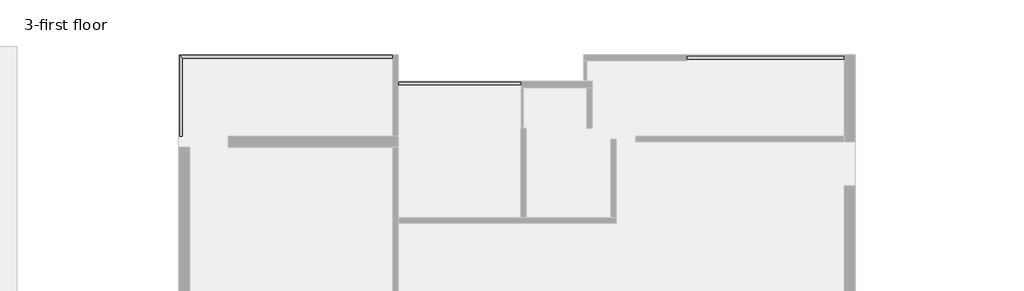
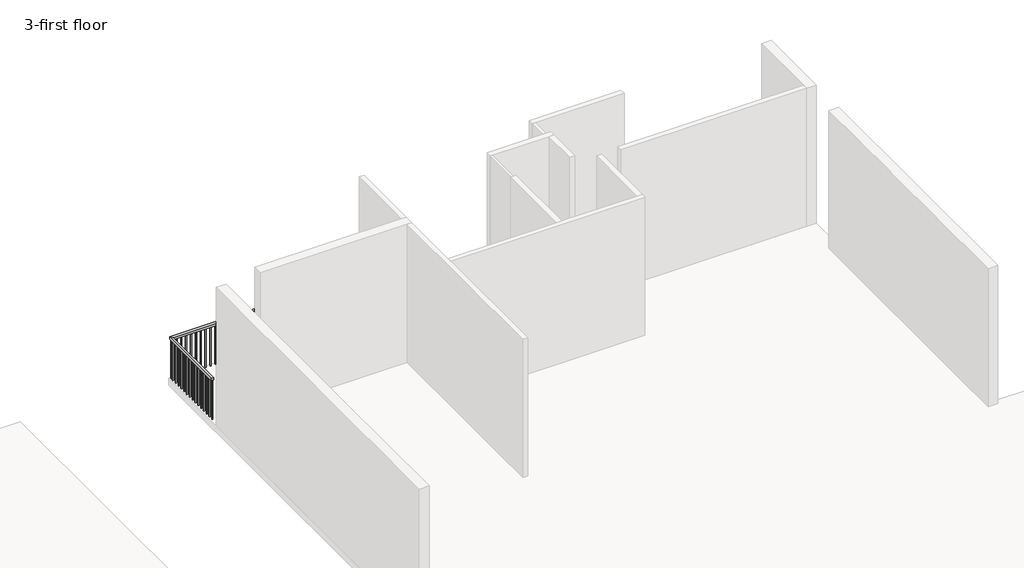
# One storey, part 2 of 2: 3 railings.
"""IFC4 building model written with IfcOpenShell, lengths in millimetres."""

from ifc_helpers import new_model, si_unit, frame, origin, place, context, project, spatial, polyline, outline, extrude, faceted_brep, element, save

model = new_model("IFC4")

# Units and contexts
model_context = context("Model", 3, world=origin())
ifc_project = project(units=[si_unit("LENGTHUNIT", "METRE", prefix="MILLI")], contexts=[model_context])

# Site, building, storey
site = spatial("IfcSite", under=ifc_project)
building = spatial("IfcBuilding", under=site)
storey = spatial("IfcBuildingStorey", under=building, Name="3-first floor", Elevation=3505.2)

# Railings
placement = place(None, origin())
element("IfcRailing", 1, ObjectType="Handrail - Rectangular", at=placement, inside=storey, context=model_context, shape_type="SolidModel", body=[
    faceted_brep([(-27068.2159189, 48850.883515, 4419.6), (-27068.2159189, 48850.883515, 4368.8), (-27017.4159189, 48850.883515, 4368.8), (-27017.4159189, 48850.883515, 4419.6), (-27017.4159189, 50306.2625405, 4368.8), (-27017.4159189, 50306.2625405, 4419.6), (-27068.2159189, 50357.0625405, 4419.6), (-23067.7159175, 50357.0625405, 4419.6), (-23067.7159175, 50306.2625405, 4419.6), (-23067.7159175, 50306.2625405, 4368.8), (-23067.7159175, 50357.0625405, 4368.8), (-27068.2159189, 50357.0625405, 4368.8)], [[[0, 1, 2, 3]], [[3, 2, 4, 5]], [[0, 3, 5, 6]], [[7, 8, 9, 10]], [[5, 4, 9, 8]], [[6, 5, 8, 7]], [[1, 0, 6, 11]], [[2, 1, 11, 4]], [[11, 6, 7, 10]], [[4, 11, 10, 9]]]),
    extrude(outline(polyline([(-23089.9409189, 50322.1375405), (-23089.9409189, 50341.1875405), (-23070.8909189, 50341.1875405), (-23070.8909189, 50322.1375405), (-23089.9409189, 50322.1375405)])), frame((0.0, 0.0, 3505.2), z_axis=(0.0, 0.0, 1.0), x_axis=(1.0, 0.0, 0.0)), (0.0, 0.0, 1.0), 863.6),
    extrude(outline(polyline([(-23191.5409189, 50322.1375405), (-23191.5409189, 50341.1875405), (-23172.4909189, 50341.1875405), (-23172.4909189, 50322.1375405), (-23191.5409189, 50322.1375405)])), frame((0.0, 0.0, 3505.2), z_axis=(0.0, 0.0, 1.0), x_axis=(1.0, 0.0, 0.0)), (0.0, 0.0, 1.0), 863.6),
    extrude(outline(polyline([(-23293.1409189, 50322.1375405), (-23293.1409189, 50341.1875405), (-23274.0909189, 50341.1875405), (-23274.0909189, 50322.1375405), (-23293.1409189, 50322.1375405)])), frame((0.0, 0.0, 3505.2), z_axis=(0.0, 0.0, 1.0), x_axis=(1.0, 0.0, 0.0)), (0.0, 0.0, 1.0), 863.6),
    extrude(outline(polyline([(-23394.7409189, 50322.1375405), (-23394.7409189, 50341.1875405), (-23375.6909189, 50341.1875405), (-23375.6909189, 50322.1375405), (-23394.7409189, 50322.1375405)])), frame((0.0, 0.0, 3505.2), z_axis=(0.0, 0.0, 1.0), x_axis=(1.0, 0.0, 0.0)), (0.0, 0.0, 1.0), 863.6),
    extrude(outline(polyline([(-23496.3409189, 50322.1375405), (-23496.3409189, 50341.1875405), (-23477.2909189, 50341.1875405), (-23477.2909189, 50322.1375405), (-23496.3409189, 50322.1375405)])), frame((0.0, 0.0, 3505.2), z_axis=(0.0, 0.0, 1.0), x_axis=(1.0, 0.0, 0.0)), (0.0, 0.0, 1.0), 863.6),
    extrude(outline(polyline([(-23597.9409189, 50322.1375405), (-23597.9409189, 50341.1875405), (-23578.8909189, 50341.1875405), (-23578.8909189, 50322.1375405), (-23597.9409189, 50322.1375405)])), frame((0.0, 0.0, 3505.2), z_axis=(0.0, 0.0, 1.0), x_axis=(1.0, 0.0, 0.0)), (0.0, 0.0, 1.0), 863.6),
    extrude(outline(polyline([(-23699.5409189, 50322.1375405), (-23699.5409189, 50341.1875405), (-23680.4909189, 50341.1875405), (-23680.4909189, 50322.1375405), (-23699.5409189, 50322.1375405)])), frame((0.0, 0.0, 3505.2), z_axis=(0.0, 0.0, 1.0), x_axis=(1.0, 0.0, 0.0)), (0.0, 0.0, 1.0), 863.6),
    extrude(outline(polyline([(-23801.1409189, 50322.1375405), (-23801.1409189, 50341.1875405), (-23782.0909189, 50341.1875405), (-23782.0909189, 50322.1375405), (-23801.1409189, 50322.1375405)])), frame((0.0, 0.0, 3505.2), z_axis=(0.0, 0.0, 1.0), x_axis=(1.0, 0.0, 0.0)), (0.0, 0.0, 1.0), 863.6),
    extrude(outline(polyline([(-23902.7409189, 50322.1375405), (-23902.7409189, 50341.1875405), (-23883.6909189, 50341.1875405), (-23883.6909189, 50322.1375405), (-23902.7409189, 50322.1375405)])), frame((0.0, 0.0, 3505.2), z_axis=(0.0, 0.0, 1.0), x_axis=(1.0, 0.0, 0.0)), (0.0, 0.0, 1.0), 863.6),
    extrude(outline(polyline([(-24004.3409189, 50322.1375405), (-24004.3409189, 50341.1875405), (-23985.2909189, 50341.1875405), (-23985.2909189, 50322.1375405), (-24004.3409189, 50322.1375405)])), frame((0.0, 0.0, 3505.2), z_axis=(0.0, 0.0, 1.0), x_axis=(1.0, 0.0, 0.0)), (0.0, 0.0, 1.0), 863.6),
    extrude(outline(polyline([(-24105.9409189, 50322.1375405), (-24105.9409189, 50341.1875405), (-24086.8909189, 50341.1875405), (-24086.8909189, 50322.1375405), (-24105.9409189, 50322.1375405)])), frame((0.0, 0.0, 3505.2), z_axis=(0.0, 0.0, 1.0), x_axis=(1.0, 0.0, 0.0)), (0.0, 0.0, 1.0), 863.6),
    extrude(outline(polyline([(-24207.5409189, 50322.1375405), (-24207.5409189, 50341.1875405), (-24188.4909189, 50341.1875405), (-24188.4909189, 50322.1375405), (-24207.5409189, 50322.1375405)])), frame((0.0, 0.0, 3505.2), z_axis=(0.0, 0.0, 1.0), x_axis=(1.0, 0.0, 0.0)), (0.0, 0.0, 1.0), 863.6),
    extrude(outline(polyline([(-24309.1409189, 50322.1375405), (-24309.1409189, 50341.1875405), (-24290.0909189, 50341.1875405), (-24290.0909189, 50322.1375405), (-24309.1409189, 50322.1375405)])), frame((0.0, 0.0, 3505.2), z_axis=(0.0, 0.0, 1.0), x_axis=(1.0, 0.0, 0.0)), (0.0, 0.0, 1.0), 863.6),
    extrude(outline(polyline([(-24410.7409189, 50322.1375405), (-24410.7409189, 50341.1875405), (-24391.6909189, 50341.1875405), (-24391.6909189, 50322.1375405), (-24410.7409189, 50322.1375405)])), frame((0.0, 0.0, 3505.2), z_axis=(0.0, 0.0, 1.0), x_axis=(1.0, 0.0, 0.0)), (0.0, 0.0, 1.0), 863.6),
    extrude(outline(polyline([(-24512.3409189, 50322.1375405), (-24512.3409189, 50341.1875405), (-24493.2909189, 50341.1875405), (-24493.2909189, 50322.1375405), (-24512.3409189, 50322.1375405)])), frame((0.0, 0.0, 3505.2), z_axis=(0.0, 0.0, 1.0), x_axis=(1.0, 0.0, 0.0)), (0.0, 0.0, 1.0), 863.6),
    extrude(outline(polyline([(-24613.9409189, 50322.1375405), (-24613.9409189, 50341.1875405), (-24594.8909189, 50341.1875405), (-24594.8909189, 50322.1375405), (-24613.9409189, 50322.1375405)])), frame((0.0, 0.0, 3505.2), z_axis=(0.0, 0.0, 1.0), x_axis=(1.0, 0.0, 0.0)), (0.0, 0.0, 1.0), 863.6),
    extrude(outline(polyline([(-24715.5409189, 50322.1375405), (-24715.5409189, 50341.1875405), (-24696.4909189, 50341.1875405), (-24696.4909189, 50322.1375405), (-24715.5409189, 50322.1375405)])), frame((0.0, 0.0, 3505.2), z_axis=(0.0, 0.0, 1.0), x_axis=(1.0, 0.0, 0.0)), (0.0, 0.0, 1.0), 863.6),
    extrude(outline(polyline([(-24817.1409189, 50322.1375405), (-24817.1409189, 50341.1875405), (-24798.0909189, 50341.1875405), (-24798.0909189, 50322.1375405), (-24817.1409189, 50322.1375405)])), frame((0.0, 0.0, 3505.2), z_axis=(0.0, 0.0, 1.0), x_axis=(1.0, 0.0, 0.0)), (0.0, 0.0, 1.0), 863.6),
    extrude(outline(polyline([(-24918.7409189, 50322.1375405), (-24918.7409189, 50341.1875405), (-24899.6909189, 50341.1875405), (-24899.6909189, 50322.1375405), (-24918.7409189, 50322.1375405)])), frame((0.0, 0.0, 3505.2), z_axis=(0.0, 0.0, 1.0), x_axis=(1.0, 0.0, 0.0)), (0.0, 0.0, 1.0), 863.6),
    extrude(outline(polyline([(-25020.3409189, 50322.1375405), (-25020.3409189, 50341.1875405), (-25001.2909189, 50341.1875405), (-25001.2909189, 50322.1375405), (-25020.3409189, 50322.1375405)])), frame((0.0, 0.0, 3505.2), z_axis=(0.0, 0.0, 1.0), x_axis=(1.0, 0.0, 0.0)), (0.0, 0.0, 1.0), 863.6),
    extrude(outline(polyline([(-25121.9409189, 50322.1375405), (-25121.9409189, 50341.1875405), (-25102.8909189, 50341.1875405), (-25102.8909189, 50322.1375405), (-25121.9409189, 50322.1375405)])), frame((0.0, 0.0, 3505.2), z_axis=(0.0, 0.0, 1.0), x_axis=(1.0, 0.0, 0.0)), (0.0, 0.0, 1.0), 863.6),
    extrude(outline(polyline([(-25223.5409189, 50322.1375405), (-25223.5409189, 50341.1875405), (-25204.4909189, 50341.1875405), (-25204.4909189, 50322.1375405), (-25223.5409189, 50322.1375405)])), frame((0.0, 0.0, 3505.2), z_axis=(0.0, 0.0, 1.0), x_axis=(1.0, 0.0, 0.0)), (0.0, 0.0, 1.0), 863.6),
    extrude(outline(polyline([(-25325.1409189, 50322.1375405), (-25325.1409189, 50341.1875405), (-25306.0909189, 50341.1875405), (-25306.0909189, 50322.1375405), (-25325.1409189, 50322.1375405)])), frame((0.0, 0.0, 3505.2), z_axis=(0.0, 0.0, 1.0), x_axis=(1.0, 0.0, 0.0)), (0.0, 0.0, 1.0), 863.6),
    extrude(outline(polyline([(-25426.7409189, 50322.1375405), (-25426.7409189, 50341.1875405), (-25407.6909189, 50341.1875405), (-25407.6909189, 50322.1375405), (-25426.7409189, 50322.1375405)])), frame((0.0, 0.0, 3505.2), z_axis=(0.0, 0.0, 1.0), x_axis=(1.0, 0.0, 0.0)), (0.0, 0.0, 1.0), 863.6),
    extrude(outline(polyline([(-25528.3409189, 50322.1375405), (-25528.3409189, 50341.1875405), (-25509.2909189, 50341.1875405), (-25509.2909189, 50322.1375405), (-25528.3409189, 50322.1375405)])), frame((0.0, 0.0, 3505.2), z_axis=(0.0, 0.0, 1.0), x_axis=(1.0, 0.0, 0.0)), (0.0, 0.0, 1.0), 863.6),
    extrude(outline(polyline([(-25629.9409189, 50322.1375405), (-25629.9409189, 50341.1875405), (-25610.8909189, 50341.1875405), (-25610.8909189, 50322.1375405), (-25629.9409189, 50322.1375405)])), frame((0.0, 0.0, 3505.2), z_axis=(0.0, 0.0, 1.0), x_axis=(1.0, 0.0, 0.0)), (0.0, 0.0, 1.0), 863.6),
    extrude(outline(polyline([(-25731.5409189, 50322.1375405), (-25731.5409189, 50341.1875405), (-25712.4909189, 50341.1875405), (-25712.4909189, 50322.1375405), (-25731.5409189, 50322.1375405)])), frame((0.0, 0.0, 3505.2), z_axis=(0.0, 0.0, 1.0), x_axis=(1.0, 0.0, 0.0)), (0.0, 0.0, 1.0), 863.6),
    extrude(outline(polyline([(-25833.1409189, 50322.1375405), (-25833.1409189, 50341.1875405), (-25814.0909189, 50341.1875405), (-25814.0909189, 50322.1375405), (-25833.1409189, 50322.1375405)])), frame((0.0, 0.0, 3505.2), z_axis=(0.0, 0.0, 1.0), x_axis=(1.0, 0.0, 0.0)), (0.0, 0.0, 1.0), 863.6),
    extrude(outline(polyline([(-25934.7409189, 50322.1375405), (-25934.7409189, 50341.1875405), (-25915.6909189, 50341.1875405), (-25915.6909189, 50322.1375405), (-25934.7409189, 50322.1375405)])), frame((0.0, 0.0, 3505.2), z_axis=(0.0, 0.0, 1.0), x_axis=(1.0, 0.0, 0.0)), (0.0, 0.0, 1.0), 863.6),
    extrude(outline(polyline([(-26036.3409189, 50322.1375405), (-26036.3409189, 50341.1875405), (-26017.2909189, 50341.1875405), (-26017.2909189, 50322.1375405), (-26036.3409189, 50322.1375405)])), frame((0.0, 0.0, 3505.2), z_axis=(0.0, 0.0, 1.0), x_axis=(1.0, 0.0, 0.0)), (0.0, 0.0, 1.0), 863.6),
    extrude(outline(polyline([(-26137.9409189, 50322.1375405), (-26137.9409189, 50341.1875405), (-26118.8909189, 50341.1875405), (-26118.8909189, 50322.1375405), (-26137.9409189, 50322.1375405)])), frame((0.0, 0.0, 3505.2), z_axis=(0.0, 0.0, 1.0), x_axis=(1.0, 0.0, 0.0)), (0.0, 0.0, 1.0), 863.6),
    extrude(outline(polyline([(-26239.5409189, 50322.1375405), (-26239.5409189, 50341.1875405), (-26220.4909189, 50341.1875405), (-26220.4909189, 50322.1375405), (-26239.5409189, 50322.1375405)])), frame((0.0, 0.0, 3505.2), z_axis=(0.0, 0.0, 1.0), x_axis=(1.0, 0.0, 0.0)), (0.0, 0.0, 1.0), 863.6),
    extrude(outline(polyline([(-26341.1409189, 50322.1375405), (-26341.1409189, 50341.1875405), (-26322.0909189, 50341.1875405), (-26322.0909189, 50322.1375405), (-26341.1409189, 50322.1375405)])), frame((0.0, 0.0, 3505.2), z_axis=(0.0, 0.0, 1.0), x_axis=(1.0, 0.0, 0.0)), (0.0, 0.0, 1.0), 863.6),
    extrude(outline(polyline([(-26442.7409189, 50322.1375405), (-26442.7409189, 50341.1875405), (-26423.6909189, 50341.1875405), (-26423.6909189, 50322.1375405), (-26442.7409189, 50322.1375405)])), frame((0.0, 0.0, 3505.2), z_axis=(0.0, 0.0, 1.0), x_axis=(1.0, 0.0, 0.0)), (0.0, 0.0, 1.0), 863.6),
    extrude(outline(polyline([(-26544.3409189, 50322.1375405), (-26544.3409189, 50341.1875405), (-26525.2909189, 50341.1875405), (-26525.2909189, 50322.1375405), (-26544.3409189, 50322.1375405)])), frame((0.0, 0.0, 3505.2), z_axis=(0.0, 0.0, 1.0), x_axis=(1.0, 0.0, 0.0)), (0.0, 0.0, 1.0), 863.6),
    extrude(outline(polyline([(-26645.9409189, 50322.1375405), (-26645.9409189, 50341.1875405), (-26626.8909189, 50341.1875405), (-26626.8909189, 50322.1375405), (-26645.9409189, 50322.1375405)])), frame((0.0, 0.0, 3505.2), z_axis=(0.0, 0.0, 1.0), x_axis=(1.0, 0.0, 0.0)), (0.0, 0.0, 1.0), 863.6),
    extrude(outline(polyline([(-26747.5409189, 50322.1375405), (-26747.5409189, 50341.1875405), (-26728.4909189, 50341.1875405), (-26728.4909189, 50322.1375405), (-26747.5409189, 50322.1375405)])), frame((0.0, 0.0, 3505.2), z_axis=(0.0, 0.0, 1.0), x_axis=(1.0, 0.0, 0.0)), (0.0, 0.0, 1.0), 863.6),
    extrude(outline(polyline([(-26849.1409189, 50322.1375405), (-26849.1409189, 50341.1875405), (-26830.0909189, 50341.1875405), (-26830.0909189, 50322.1375405), (-26849.1409189, 50322.1375405)])), frame((0.0, 0.0, 3505.2), z_axis=(0.0, 0.0, 1.0), x_axis=(1.0, 0.0, 0.0)), (0.0, 0.0, 1.0), 863.6),
    extrude(outline(polyline([(-26950.7409189, 50322.1375405), (-26950.7409189, 50341.1875405), (-26931.6909189, 50341.1875405), (-26931.6909189, 50322.1375405), (-26950.7409189, 50322.1375405)])), frame((0.0, 0.0, 3505.2), z_axis=(0.0, 0.0, 1.0), x_axis=(1.0, 0.0, 0.0)), (0.0, 0.0, 1.0), 863.6),
    extrude(outline(polyline([(-27033.2909189, 50263.758515), (-27052.3409189, 50263.758515), (-27052.3409189, 50282.808515), (-27033.2909189, 50282.808515), (-27033.2909189, 50263.758515)])), frame((0.0, 0.0, 3505.2), z_axis=(0.0, 0.0, 1.0), x_axis=(1.0, 0.0, 0.0)), (0.0, 0.0, 1.0), 863.6),
    extrude(outline(polyline([(-27033.2909189, 50162.158515), (-27052.3409189, 50162.158515), (-27052.3409189, 50181.208515), (-27033.2909189, 50181.208515), (-27033.2909189, 50162.158515)])), frame((0.0, 0.0, 3505.2), z_axis=(0.0, 0.0, 1.0), x_axis=(1.0, 0.0, 0.0)), (0.0, 0.0, 1.0), 863.6),
    extrude(outline(polyline([(-27033.2909189, 50060.558515), (-27052.3409189, 50060.558515), (-27052.3409189, 50079.608515), (-27033.2909189, 50079.608515), (-27033.2909189, 50060.558515)])), frame((0.0, 0.0, 3505.2), z_axis=(0.0, 0.0, 1.0), x_axis=(1.0, 0.0, 0.0)), (0.0, 0.0, 1.0), 863.6),
    extrude(outline(polyline([(-27033.2909189, 49958.958515), (-27052.3409189, 49958.958515), (-27052.3409189, 49978.008515), (-27033.2909189, 49978.008515), (-27033.2909189, 49958.958515)])), frame((0.0, 0.0, 3505.2), z_axis=(0.0, 0.0, 1.0), x_axis=(1.0, 0.0, 0.0)), (0.0, 0.0, 1.0), 863.6),
    extrude(outline(polyline([(-27033.2909189, 49857.358515), (-27052.3409189, 49857.358515), (-27052.3409189, 49876.408515), (-27033.2909189, 49876.408515), (-27033.2909189, 49857.358515)])), frame((0.0, 0.0, 3505.2), z_axis=(0.0, 0.0, 1.0), x_axis=(1.0, 0.0, 0.0)), (0.0, 0.0, 1.0), 863.6),
    extrude(outline(polyline([(-27033.2909189, 49755.758515), (-27052.3409189, 49755.758515), (-27052.3409189, 49774.808515), (-27033.2909189, 49774.808515), (-27033.2909189, 49755.758515)])), frame((0.0, 0.0, 3505.2), z_axis=(0.0, 0.0, 1.0), x_axis=(1.0, 0.0, 0.0)), (0.0, 0.0, 1.0), 863.6),
    extrude(outline(polyline([(-27033.2909189, 49654.158515), (-27052.3409189, 49654.158515), (-27052.3409189, 49673.208515), (-27033.2909189, 49673.208515), (-27033.2909189, 49654.158515)])), frame((0.0, 0.0, 3505.2), z_axis=(0.0, 0.0, 1.0), x_axis=(1.0, 0.0, 0.0)), (0.0, 0.0, 1.0), 863.6),
    extrude(outline(polyline([(-27033.2909189, 49552.558515), (-27052.3409189, 49552.558515), (-27052.3409189, 49571.608515), (-27033.2909189, 49571.608515), (-27033.2909189, 49552.558515)])), frame((0.0, 0.0, 3505.2), z_axis=(0.0, 0.0, 1.0), x_axis=(1.0, 0.0, 0.0)), (0.0, 0.0, 1.0), 863.6),
    extrude(outline(polyline([(-27033.2909189, 49450.958515), (-27052.3409189, 49450.958515), (-27052.3409189, 49470.008515), (-27033.2909189, 49470.008515), (-27033.2909189, 49450.958515)])), frame((0.0, 0.0, 3505.2), z_axis=(0.0, 0.0, 1.0), x_axis=(1.0, 0.0, 0.0)), (0.0, 0.0, 1.0), 863.6),
    extrude(outline(polyline([(-27033.2909189, 49349.358515), (-27052.3409189, 49349.358515), (-27052.3409189, 49368.408515), (-27033.2909189, 49368.408515), (-27033.2909189, 49349.358515)])), frame((0.0, 0.0, 3505.2), z_axis=(0.0, 0.0, 1.0), x_axis=(1.0, 0.0, 0.0)), (0.0, 0.0, 1.0), 863.6),
    extrude(outline(polyline([(-27033.2909189, 49247.758515), (-27052.3409189, 49247.758515), (-27052.3409189, 49266.808515), (-27033.2909189, 49266.808515), (-27033.2909189, 49247.758515)])), frame((0.0, 0.0, 3505.2), z_axis=(0.0, 0.0, 1.0), x_axis=(1.0, 0.0, 0.0)), (0.0, 0.0, 1.0), 863.6),
    extrude(outline(polyline([(-27033.2909189, 49146.158515), (-27052.3409189, 49146.158515), (-27052.3409189, 49165.208515), (-27033.2909189, 49165.208515), (-27033.2909189, 49146.158515)])), frame((0.0, 0.0, 3505.2), z_axis=(0.0, 0.0, 1.0), x_axis=(1.0, 0.0, 0.0)), (0.0, 0.0, 1.0), 863.6),
    extrude(outline(polyline([(-27033.2909189, 49044.558515), (-27052.3409189, 49044.558515), (-27052.3409189, 49063.608515), (-27033.2909189, 49063.608515), (-27033.2909189, 49044.558515)])), frame((0.0, 0.0, 3505.2), z_axis=(0.0, 0.0, 1.0), x_axis=(1.0, 0.0, 0.0)), (0.0, 0.0, 1.0), 863.6),
    extrude(outline(polyline([(-27033.2909189, 48942.958515), (-27052.3409189, 48942.958515), (-27052.3409189, 48962.008515), (-27033.2909189, 48962.008515), (-27033.2909189, 48942.958515)])), frame((0.0, 0.0, 3505.2), z_axis=(0.0, 0.0, 1.0), x_axis=(1.0, 0.0, 0.0)), (0.0, 0.0, 1.0), 863.6),
    extrude(outline(polyline([(-27033.2909189, 50322.1375405), (-27052.3409189, 50322.1375405), (-27052.3409189, 50341.1875405), (-27033.2909189, 50341.1875405), (-27033.2909189, 50322.1375405)])), frame((0.0, 0.0, 3505.2), z_axis=(0.0, 0.0, 1.0), x_axis=(1.0, 0.0, 0.0)), (0.0, 0.0, 1.0), 863.6),
    extrude(outline(polyline([(-23086.7659175, 50322.1375405), (-23086.7659175, 50341.1875405), (-23067.7159175, 50341.1875405), (-23067.7159175, 50322.1375405), (-23086.7659175, 50322.1375405)])), frame((0.0, 0.0, 3505.2), z_axis=(0.0, 0.0, 1.0), x_axis=(1.0, 0.0, 0.0)), (0.0, 0.0, 1.0), 863.6),
    extrude(outline(polyline([(-27033.2909189, 48850.883515), (-27052.3409189, 48850.883515), (-27052.3409189, 48869.933515), (-27033.2909189, 48869.933515), (-27033.2909189, 48850.883515)])), frame((0.0, 0.0, 3505.2), z_axis=(0.0, 0.0, 1.0), x_axis=(1.0, 0.0, 0.0)), (0.0, 0.0, 1.0), 863.6),
])
element("IfcRailing", 2, ObjectType="Handrail - Rectangular", at=placement, inside=storey, context=model_context, shape_type="SweptSolid", body=[
    extrude(outline(polyline([(-23004.2159175, 49810.9625405), (-23004.2159175, 49861.7625405), (-20721.5933155, 49861.7625405), (-20721.5933155, 49810.9625405), (-23004.2159175, 49810.9625405)])), frame((0.0, 0.0, 4368.8), z_axis=(0.0, 0.0, 1.0), x_axis=(1.0, 0.0, 0.0)), (0.0, 0.0, 1.0), 50.8),
    extrude(outline(polyline([(-20778.5409175, 49826.8375405), (-20778.5409175, 49845.8875405), (-20759.4909175, 49845.8875405), (-20759.4909175, 49826.8375405), (-20778.5409175, 49826.8375405)])), frame((0.0, 0.0, 3505.2), z_axis=(0.0, 0.0, 1.0), x_axis=(1.0, 0.0, 0.0)), (0.0, 0.0, 1.0), 863.6),
    extrude(outline(polyline([(-20880.1409175, 49826.8375405), (-20880.1409175, 49845.8875405), (-20861.0909175, 49845.8875405), (-20861.0909175, 49826.8375405), (-20880.1409175, 49826.8375405)])), frame((0.0, 0.0, 3505.2), z_axis=(0.0, 0.0, 1.0), x_axis=(1.0, 0.0, 0.0)), (0.0, 0.0, 1.0), 863.6),
    extrude(outline(polyline([(-20981.7409175, 49826.8375405), (-20981.7409175, 49845.8875405), (-20962.6909175, 49845.8875405), (-20962.6909175, 49826.8375405), (-20981.7409175, 49826.8375405)])), frame((0.0, 0.0, 3505.2), z_axis=(0.0, 0.0, 1.0), x_axis=(1.0, 0.0, 0.0)), (0.0, 0.0, 1.0), 863.6),
    extrude(outline(polyline([(-21083.3409175, 49826.8375405), (-21083.3409175, 49845.8875405), (-21064.2909175, 49845.8875405), (-21064.2909175, 49826.8375405), (-21083.3409175, 49826.8375405)])), frame((0.0, 0.0, 3505.2), z_axis=(0.0, 0.0, 1.0), x_axis=(1.0, 0.0, 0.0)), (0.0, 0.0, 1.0), 863.6),
    extrude(outline(polyline([(-21184.9409175, 49826.8375405), (-21184.9409175, 49845.8875405), (-21165.8909175, 49845.8875405), (-21165.8909175, 49826.8375405), (-21184.9409175, 49826.8375405)])), frame((0.0, 0.0, 3505.2), z_axis=(0.0, 0.0, 1.0), x_axis=(1.0, 0.0, 0.0)), (0.0, 0.0, 1.0), 863.6),
    extrude(outline(polyline([(-21286.5409175, 49826.8375405), (-21286.5409175, 49845.8875405), (-21267.4909175, 49845.8875405), (-21267.4909175, 49826.8375405), (-21286.5409175, 49826.8375405)])), frame((0.0, 0.0, 3505.2), z_axis=(0.0, 0.0, 1.0), x_axis=(1.0, 0.0, 0.0)), (0.0, 0.0, 1.0), 863.6),
    extrude(outline(polyline([(-21388.1409175, 49826.8375405), (-21388.1409175, 49845.8875405), (-21369.0909175, 49845.8875405), (-21369.0909175, 49826.8375405), (-21388.1409175, 49826.8375405)])), frame((0.0, 0.0, 3505.2), z_axis=(0.0, 0.0, 1.0), x_axis=(1.0, 0.0, 0.0)), (0.0, 0.0, 1.0), 863.6),
    extrude(outline(polyline([(-21489.7409175, 49826.8375405), (-21489.7409175, 49845.8875405), (-21470.6909175, 49845.8875405), (-21470.6909175, 49826.8375405), (-21489.7409175, 49826.8375405)])), frame((0.0, 0.0, 3505.2), z_axis=(0.0, 0.0, 1.0), x_axis=(1.0, 0.0, 0.0)), (0.0, 0.0, 1.0), 863.6),
    extrude(outline(polyline([(-21591.3409175, 49826.8375405), (-21591.3409175, 49845.8875405), (-21572.2909175, 49845.8875405), (-21572.2909175, 49826.8375405), (-21591.3409175, 49826.8375405)])), frame((0.0, 0.0, 3505.2), z_axis=(0.0, 0.0, 1.0), x_axis=(1.0, 0.0, 0.0)), (0.0, 0.0, 1.0), 863.6),
    extrude(outline(polyline([(-21692.9409175, 49826.8375405), (-21692.9409175, 49845.8875405), (-21673.8909175, 49845.8875405), (-21673.8909175, 49826.8375405), (-21692.9409175, 49826.8375405)])), frame((0.0, 0.0, 3505.2), z_axis=(0.0, 0.0, 1.0), x_axis=(1.0, 0.0, 0.0)), (0.0, 0.0, 1.0), 863.6),
    extrude(outline(polyline([(-21794.5409175, 49826.8375405), (-21794.5409175, 49845.8875405), (-21775.4909175, 49845.8875405), (-21775.4909175, 49826.8375405), (-21794.5409175, 49826.8375405)])), frame((0.0, 0.0, 3505.2), z_axis=(0.0, 0.0, 1.0), x_axis=(1.0, 0.0, 0.0)), (0.0, 0.0, 1.0), 863.6),
    extrude(outline(polyline([(-21896.1409175, 49826.8375405), (-21896.1409175, 49845.8875405), (-21877.0909175, 49845.8875405), (-21877.0909175, 49826.8375405), (-21896.1409175, 49826.8375405)])), frame((0.0, 0.0, 3505.2), z_axis=(0.0, 0.0, 1.0), x_axis=(1.0, 0.0, 0.0)), (0.0, 0.0, 1.0), 863.6),
    extrude(outline(polyline([(-21997.7409175, 49826.8375405), (-21997.7409175, 49845.8875405), (-21978.6909175, 49845.8875405), (-21978.6909175, 49826.8375405), (-21997.7409175, 49826.8375405)])), frame((0.0, 0.0, 3505.2), z_axis=(0.0, 0.0, 1.0), x_axis=(1.0, 0.0, 0.0)), (0.0, 0.0, 1.0), 863.6),
    extrude(outline(polyline([(-22099.3409175, 49826.8375405), (-22099.3409175, 49845.8875405), (-22080.2909175, 49845.8875405), (-22080.2909175, 49826.8375405), (-22099.3409175, 49826.8375405)])), frame((0.0, 0.0, 3505.2), z_axis=(0.0, 0.0, 1.0), x_axis=(1.0, 0.0, 0.0)), (0.0, 0.0, 1.0), 863.6),
    extrude(outline(polyline([(-22200.9409175, 49826.8375405), (-22200.9409175, 49845.8875405), (-22181.8909175, 49845.8875405), (-22181.8909175, 49826.8375405), (-22200.9409175, 49826.8375405)])), frame((0.0, 0.0, 3505.2), z_axis=(0.0, 0.0, 1.0), x_axis=(1.0, 0.0, 0.0)), (0.0, 0.0, 1.0), 863.6),
    extrude(outline(polyline([(-22302.5409175, 49826.8375405), (-22302.5409175, 49845.8875405), (-22283.4909175, 49845.8875405), (-22283.4909175, 49826.8375405), (-22302.5409175, 49826.8375405)])), frame((0.0, 0.0, 3505.2), z_axis=(0.0, 0.0, 1.0), x_axis=(1.0, 0.0, 0.0)), (0.0, 0.0, 1.0), 863.6),
    extrude(outline(polyline([(-22404.1409175, 49826.8375405), (-22404.1409175, 49845.8875405), (-22385.0909175, 49845.8875405), (-22385.0909175, 49826.8375405), (-22404.1409175, 49826.8375405)])), frame((0.0, 0.0, 3505.2), z_axis=(0.0, 0.0, 1.0), x_axis=(1.0, 0.0, 0.0)), (0.0, 0.0, 1.0), 863.6),
    extrude(outline(polyline([(-22505.7409175, 49826.8375405), (-22505.7409175, 49845.8875405), (-22486.6909175, 49845.8875405), (-22486.6909175, 49826.8375405), (-22505.7409175, 49826.8375405)])), frame((0.0, 0.0, 3505.2), z_axis=(0.0, 0.0, 1.0), x_axis=(1.0, 0.0, 0.0)), (0.0, 0.0, 1.0), 863.6),
    extrude(outline(polyline([(-22607.3409175, 49826.8375405), (-22607.3409175, 49845.8875405), (-22588.2909175, 49845.8875405), (-22588.2909175, 49826.8375405), (-22607.3409175, 49826.8375405)])), frame((0.0, 0.0, 3505.2), z_axis=(0.0, 0.0, 1.0), x_axis=(1.0, 0.0, 0.0)), (0.0, 0.0, 1.0), 863.6),
    extrude(outline(polyline([(-22708.9409175, 49826.8375405), (-22708.9409175, 49845.8875405), (-22689.8909175, 49845.8875405), (-22689.8909175, 49826.8375405), (-22708.9409175, 49826.8375405)])), frame((0.0, 0.0, 3505.2), z_axis=(0.0, 0.0, 1.0), x_axis=(1.0, 0.0, 0.0)), (0.0, 0.0, 1.0), 863.6),
    extrude(outline(polyline([(-22810.5409175, 49826.8375405), (-22810.5409175, 49845.8875405), (-22791.4909175, 49845.8875405), (-22791.4909175, 49826.8375405), (-22810.5409175, 49826.8375405)])), frame((0.0, 0.0, 3505.2), z_axis=(0.0, 0.0, 1.0), x_axis=(1.0, 0.0, 0.0)), (0.0, 0.0, 1.0), 863.6),
    extrude(outline(polyline([(-22912.1409175, 49826.8375405), (-22912.1409175, 49845.8875405), (-22893.0909175, 49845.8875405), (-22893.0909175, 49826.8375405), (-22912.1409175, 49826.8375405)])), frame((0.0, 0.0, 3505.2), z_axis=(0.0, 0.0, 1.0), x_axis=(1.0, 0.0, 0.0)), (0.0, 0.0, 1.0), 863.6),
    extrude(outline(polyline([(-20740.6433155, 49826.8375405), (-20740.6433155, 49845.8875405), (-20721.5933155, 49845.8875405), (-20721.5933155, 49826.8375405), (-20740.6433155, 49826.8375405)])), frame((0.0, 0.0, 3505.2), z_axis=(0.0, 0.0, 1.0), x_axis=(1.0, 0.0, 0.0)), (0.0, 0.0, 1.0), 863.6),
    extrude(outline(polyline([(-23004.2159175, 49826.8375405), (-23004.2159175, 49845.8875405), (-22985.1659175, 49845.8875405), (-22985.1659175, 49826.8375405), (-23004.2159175, 49826.8375405)])), frame((0.0, 0.0, 3505.2), z_axis=(0.0, 0.0, 1.0), x_axis=(1.0, 0.0, 0.0)), (0.0, 0.0, 1.0), 863.6),
])
element("IfcRailing", 3, ObjectType="Handrail - Rectangular", at=placement, inside=storey, context=model_context, shape_type="SweptSolid", body=[
    extrude(outline(polyline([(-17647.6473751, 50287.2125405), (-17647.6473751, 50338.0125405), (-14713.9473752, 50338.0125405), (-14713.9473752, 50287.2125405), (-17647.6473751, 50287.2125405)])), frame((0.0, 0.0, 4368.8), z_axis=(0.0, 0.0, 1.0), x_axis=(1.0, 0.0, 0.0)), (0.0, 0.0, 1.0), 50.8),
    extrude(outline(polyline([(-14812.3723751, 50303.0875405), (-14812.3723751, 50322.1375405), (-14793.3223751, 50322.1375405), (-14793.3223751, 50303.0875405), (-14812.3723751, 50303.0875405)])), frame((0.0, 0.0, 3505.2), z_axis=(0.0, 0.0, 1.0), x_axis=(1.0, 0.0, 0.0)), (0.0, 0.0, 1.0), 863.6),
    extrude(outline(polyline([(-14913.9723751, 50303.0875405), (-14913.9723751, 50322.1375405), (-14894.9223751, 50322.1375405), (-14894.9223751, 50303.0875405), (-14913.9723751, 50303.0875405)])), frame((0.0, 0.0, 3505.2), z_axis=(0.0, 0.0, 1.0), x_axis=(1.0, 0.0, 0.0)), (0.0, 0.0, 1.0), 863.6),
    extrude(outline(polyline([(-15015.5723751, 50303.0875405), (-15015.5723751, 50322.1375405), (-14996.5223751, 50322.1375405), (-14996.5223751, 50303.0875405), (-15015.5723751, 50303.0875405)])), frame((0.0, 0.0, 3505.2), z_axis=(0.0, 0.0, 1.0), x_axis=(1.0, 0.0, 0.0)), (0.0, 0.0, 1.0), 863.6),
    extrude(outline(polyline([(-15117.1723751, 50303.0875405), (-15117.1723751, 50322.1375405), (-15098.1223751, 50322.1375405), (-15098.1223751, 50303.0875405), (-15117.1723751, 50303.0875405)])), frame((0.0, 0.0, 3505.2), z_axis=(0.0, 0.0, 1.0), x_axis=(1.0, 0.0, 0.0)), (0.0, 0.0, 1.0), 863.6),
    extrude(outline(polyline([(-15218.7723751, 50303.0875405), (-15218.7723751, 50322.1375405), (-15199.7223751, 50322.1375405), (-15199.7223751, 50303.0875405), (-15218.7723751, 50303.0875405)])), frame((0.0, 0.0, 3505.2), z_axis=(0.0, 0.0, 1.0), x_axis=(1.0, 0.0, 0.0)), (0.0, 0.0, 1.0), 863.6),
    extrude(outline(polyline([(-15320.3723751, 50303.0875405), (-15320.3723751, 50322.1375405), (-15301.3223751, 50322.1375405), (-15301.3223751, 50303.0875405), (-15320.3723751, 50303.0875405)])), frame((0.0, 0.0, 3505.2), z_axis=(0.0, 0.0, 1.0), x_axis=(1.0, 0.0, 0.0)), (0.0, 0.0, 1.0), 863.6),
    extrude(outline(polyline([(-15421.9723751, 50303.0875405), (-15421.9723751, 50322.1375405), (-15402.9223751, 50322.1375405), (-15402.9223751, 50303.0875405), (-15421.9723751, 50303.0875405)])), frame((0.0, 0.0, 3505.2), z_axis=(0.0, 0.0, 1.0), x_axis=(1.0, 0.0, 0.0)), (0.0, 0.0, 1.0), 863.6),
    extrude(outline(polyline([(-15523.5723751, 50303.0875405), (-15523.5723751, 50322.1375405), (-15504.5223751, 50322.1375405), (-15504.5223751, 50303.0875405), (-15523.5723751, 50303.0875405)])), frame((0.0, 0.0, 3505.2), z_axis=(0.0, 0.0, 1.0), x_axis=(1.0, 0.0, 0.0)), (0.0, 0.0, 1.0), 863.6),
    extrude(outline(polyline([(-15625.1723751, 50303.0875405), (-15625.1723751, 50322.1375405), (-15606.1223751, 50322.1375405), (-15606.1223751, 50303.0875405), (-15625.1723751, 50303.0875405)])), frame((0.0, 0.0, 3505.2), z_axis=(0.0, 0.0, 1.0), x_axis=(1.0, 0.0, 0.0)), (0.0, 0.0, 1.0), 863.6),
    extrude(outline(polyline([(-15726.7723751, 50303.0875405), (-15726.7723751, 50322.1375405), (-15707.7223751, 50322.1375405), (-15707.7223751, 50303.0875405), (-15726.7723751, 50303.0875405)])), frame((0.0, 0.0, 3505.2), z_axis=(0.0, 0.0, 1.0), x_axis=(1.0, 0.0, 0.0)), (0.0, 0.0, 1.0), 863.6),
    extrude(outline(polyline([(-15828.3723751, 50303.0875405), (-15828.3723751, 50322.1375405), (-15809.3223751, 50322.1375405), (-15809.3223751, 50303.0875405), (-15828.3723751, 50303.0875405)])), frame((0.0, 0.0, 3505.2), z_axis=(0.0, 0.0, 1.0), x_axis=(1.0, 0.0, 0.0)), (0.0, 0.0, 1.0), 863.6),
    extrude(outline(polyline([(-15929.9723751, 50303.0875405), (-15929.9723751, 50322.1375405), (-15910.9223751, 50322.1375405), (-15910.9223751, 50303.0875405), (-15929.9723751, 50303.0875405)])), frame((0.0, 0.0, 3505.2), z_axis=(0.0, 0.0, 1.0), x_axis=(1.0, 0.0, 0.0)), (0.0, 0.0, 1.0), 863.6),
    extrude(outline(polyline([(-16031.5723751, 50303.0875405), (-16031.5723751, 50322.1375405), (-16012.5223751, 50322.1375405), (-16012.5223751, 50303.0875405), (-16031.5723751, 50303.0875405)])), frame((0.0, 0.0, 3505.2), z_axis=(0.0, 0.0, 1.0), x_axis=(1.0, 0.0, 0.0)), (0.0, 0.0, 1.0), 863.6),
    extrude(outline(polyline([(-16133.1723751, 50303.0875405), (-16133.1723751, 50322.1375405), (-16114.1223751, 50322.1375405), (-16114.1223751, 50303.0875405), (-16133.1723751, 50303.0875405)])), frame((0.0, 0.0, 3505.2), z_axis=(0.0, 0.0, 1.0), x_axis=(1.0, 0.0, 0.0)), (0.0, 0.0, 1.0), 863.6),
    extrude(outline(polyline([(-16234.7723751, 50303.0875405), (-16234.7723751, 50322.1375405), (-16215.7223751, 50322.1375405), (-16215.7223751, 50303.0875405), (-16234.7723751, 50303.0875405)])), frame((0.0, 0.0, 3505.2), z_axis=(0.0, 0.0, 1.0), x_axis=(1.0, 0.0, 0.0)), (0.0, 0.0, 1.0), 863.6),
    extrude(outline(polyline([(-16336.3723751, 50303.0875405), (-16336.3723751, 50322.1375405), (-16317.3223751, 50322.1375405), (-16317.3223751, 50303.0875405), (-16336.3723751, 50303.0875405)])), frame((0.0, 0.0, 3505.2), z_axis=(0.0, 0.0, 1.0), x_axis=(1.0, 0.0, 0.0)), (0.0, 0.0, 1.0), 863.6),
    extrude(outline(polyline([(-16437.9723751, 50303.0875405), (-16437.9723751, 50322.1375405), (-16418.9223751, 50322.1375405), (-16418.9223751, 50303.0875405), (-16437.9723751, 50303.0875405)])), frame((0.0, 0.0, 3505.2), z_axis=(0.0, 0.0, 1.0), x_axis=(1.0, 0.0, 0.0)), (0.0, 0.0, 1.0), 863.6),
    extrude(outline(polyline([(-16539.5723751, 50303.0875405), (-16539.5723751, 50322.1375405), (-16520.5223751, 50322.1375405), (-16520.5223751, 50303.0875405), (-16539.5723751, 50303.0875405)])), frame((0.0, 0.0, 3505.2), z_axis=(0.0, 0.0, 1.0), x_axis=(1.0, 0.0, 0.0)), (0.0, 0.0, 1.0), 863.6),
    extrude(outline(polyline([(-16641.1723751, 50303.0875405), (-16641.1723751, 50322.1375405), (-16622.1223751, 50322.1375405), (-16622.1223751, 50303.0875405), (-16641.1723751, 50303.0875405)])), frame((0.0, 0.0, 3505.2), z_axis=(0.0, 0.0, 1.0), x_axis=(1.0, 0.0, 0.0)), (0.0, 0.0, 1.0), 863.6),
    extrude(outline(polyline([(-16742.7723751, 50303.0875405), (-16742.7723751, 50322.1375405), (-16723.7223751, 50322.1375405), (-16723.7223751, 50303.0875405), (-16742.7723751, 50303.0875405)])), frame((0.0, 0.0, 3505.2), z_axis=(0.0, 0.0, 1.0), x_axis=(1.0, 0.0, 0.0)), (0.0, 0.0, 1.0), 863.6),
    extrude(outline(polyline([(-16844.3723751, 50303.0875405), (-16844.3723751, 50322.1375405), (-16825.3223751, 50322.1375405), (-16825.3223751, 50303.0875405), (-16844.3723751, 50303.0875405)])), frame((0.0, 0.0, 3505.2), z_axis=(0.0, 0.0, 1.0), x_axis=(1.0, 0.0, 0.0)), (0.0, 0.0, 1.0), 863.6),
    extrude(outline(polyline([(-16945.9723751, 50303.0875405), (-16945.9723751, 50322.1375405), (-16926.9223751, 50322.1375405), (-16926.9223751, 50303.0875405), (-16945.9723751, 50303.0875405)])), frame((0.0, 0.0, 3505.2), z_axis=(0.0, 0.0, 1.0), x_axis=(1.0, 0.0, 0.0)), (0.0, 0.0, 1.0), 863.6),
    extrude(outline(polyline([(-17047.5723751, 50303.0875405), (-17047.5723751, 50322.1375405), (-17028.5223751, 50322.1375405), (-17028.5223751, 50303.0875405), (-17047.5723751, 50303.0875405)])), frame((0.0, 0.0, 3505.2), z_axis=(0.0, 0.0, 1.0), x_axis=(1.0, 0.0, 0.0)), (0.0, 0.0, 1.0), 863.6),
    extrude(outline(polyline([(-17149.1723751, 50303.0875405), (-17149.1723751, 50322.1375405), (-17130.1223751, 50322.1375405), (-17130.1223751, 50303.0875405), (-17149.1723751, 50303.0875405)])), frame((0.0, 0.0, 3505.2), z_axis=(0.0, 0.0, 1.0), x_axis=(1.0, 0.0, 0.0)), (0.0, 0.0, 1.0), 863.6),
    extrude(outline(polyline([(-17250.7723751, 50303.0875405), (-17250.7723751, 50322.1375405), (-17231.7223751, 50322.1375405), (-17231.7223751, 50303.0875405), (-17250.7723751, 50303.0875405)])), frame((0.0, 0.0, 3505.2), z_axis=(0.0, 0.0, 1.0), x_axis=(1.0, 0.0, 0.0)), (0.0, 0.0, 1.0), 863.6),
    extrude(outline(polyline([(-17352.3723751, 50303.0875405), (-17352.3723751, 50322.1375405), (-17333.3223751, 50322.1375405), (-17333.3223751, 50303.0875405), (-17352.3723751, 50303.0875405)])), frame((0.0, 0.0, 3505.2), z_axis=(0.0, 0.0, 1.0), x_axis=(1.0, 0.0, 0.0)), (0.0, 0.0, 1.0), 863.6),
    extrude(outline(polyline([(-17453.9723751, 50303.0875405), (-17453.9723751, 50322.1375405), (-17434.9223751, 50322.1375405), (-17434.9223751, 50303.0875405), (-17453.9723751, 50303.0875405)])), frame((0.0, 0.0, 3505.2), z_axis=(0.0, 0.0, 1.0), x_axis=(1.0, 0.0, 0.0)), (0.0, 0.0, 1.0), 863.6),
    extrude(outline(polyline([(-17555.5723751, 50303.0875405), (-17555.5723751, 50322.1375405), (-17536.5223751, 50322.1375405), (-17536.5223751, 50303.0875405), (-17555.5723751, 50303.0875405)])), frame((0.0, 0.0, 3505.2), z_axis=(0.0, 0.0, 1.0), x_axis=(1.0, 0.0, 0.0)), (0.0, 0.0, 1.0), 863.6),
    extrude(outline(polyline([(-14732.9973752, 50303.0875405), (-14732.9973752, 50322.1375405), (-14713.9473752, 50322.1375405), (-14713.9473752, 50303.0875405), (-14732.9973752, 50303.0875405)])), frame((0.0, 0.0, 3505.2), z_axis=(0.0, 0.0, 1.0), x_axis=(1.0, 0.0, 0.0)), (0.0, 0.0, 1.0), 863.6),
    extrude(outline(polyline([(-17647.6473751, 50303.0875405), (-17647.6473751, 50322.1375405), (-17628.5973751, 50322.1375405), (-17628.5973751, 50303.0875405), (-17647.6473751, 50303.0875405)])), frame((0.0, 0.0, 3505.2), z_axis=(0.0, 0.0, 1.0), x_axis=(1.0, 0.0, 0.0)), (0.0, 0.0, 1.0), 863.6),
])

save(model, "model.ifc")

# Revit data of these elements
# Type "Handrail - Rectangular"
#   Assembly Code = "C2010400"
#   built-in parameter 1008612 = 0.0416667 (stored number, unit not read)
#   built-in parameter 1008611 = 0.0416667 (stored number, unit not read)
#   built-in parameter 1008609 = 0.333333 (stored number, unit not read)
#   built-in parameter 1008604 = 0.166667 (stored number, unit not read)
#   built-in parameter 1008603 = 0.166667 (stored number, unit not read)
#   Railing Height = 3' - 0"
#   built-in parameter 1008630 = 2
#   built-in parameter 1008610 = 2
#   built-in parameter 1008618 = Baluster - Square : 3/4"
# Elements 1, 2, 3 (IfcRailing, "Handrail - Rectangular")
#   Phase Created = New Construction
